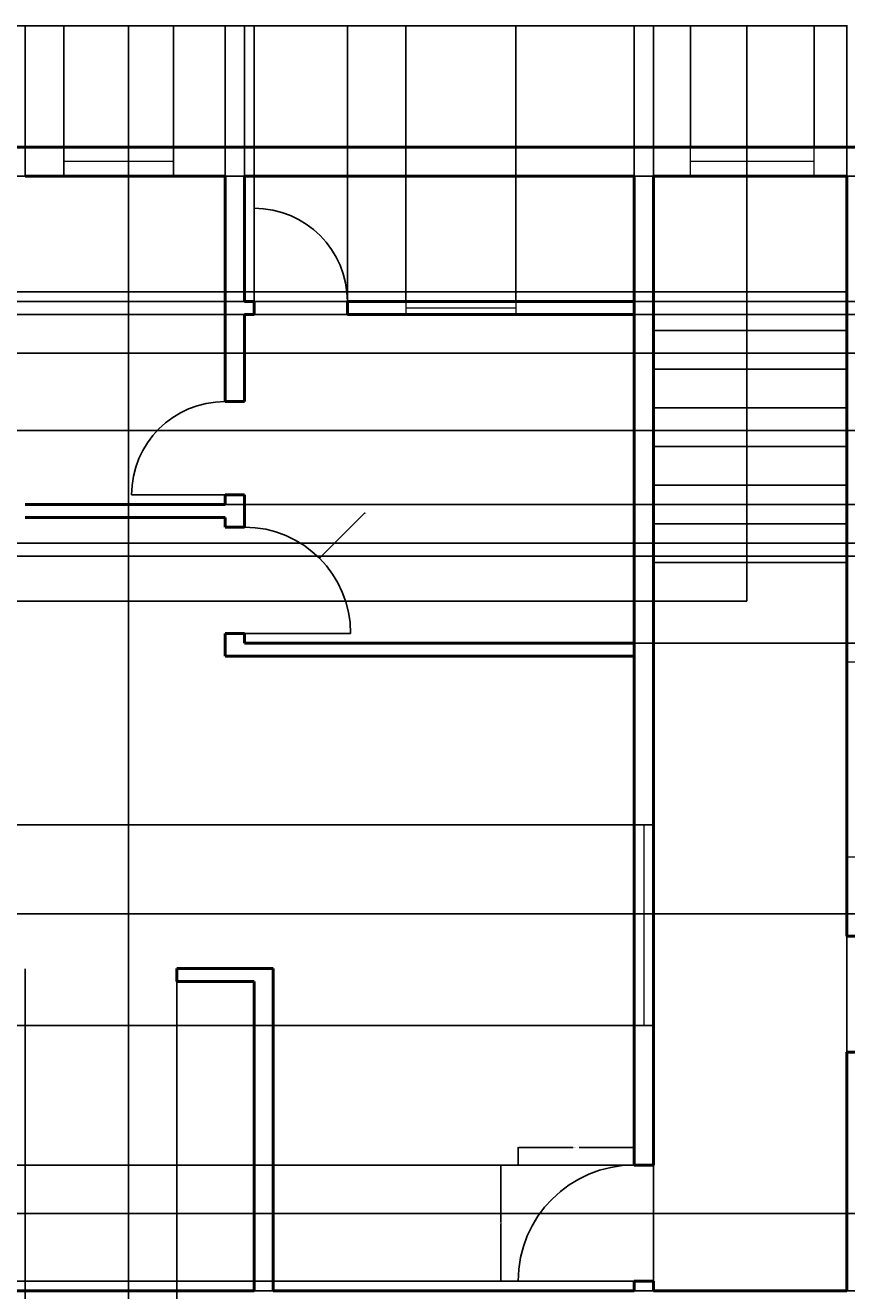
# Model space of a CAD drawing. Units: inches. Extents: x 2479 to 3284, y 2154 to 2936.
# Tile 4 of 8: x 2650 to 2905, y 2543 to 2936. Entities that reach past the tile are written whole.
import ezdxf

# ---------------------------------------------------------------- set-up
doc = ezdxf.new("R2010")
doc.units = ezdxf.units.IN
for name, color, linetype, lineweight in [('A-ANNO-DIMS', 2, 'Continuous', 18), ('A-DOOR', 3, 'Continuous', 25), ('A-FLOR-CASE', 8, 'Continuous', 18), ('A-FLOR-STRS', 2, 'Continuous', 25), ('A-GLAZ', 4, 'Continuous', 18), ('A-WALL', 7, 'Continuous', 50)]:
    doc.layers.add(name, color=color, linetype=linetype, lineweight=lineweight)
doc.styles.get("Standard").update_dxf_attribs({"font": 'arial.ttf'})
doc.dimstyles.get("Standard").update_dxf_attribs({"dimtxt": 0.18, "dimasz": 0.18, "dimexe": 0.18, "dimexo": 0.0625, "dimgap": 0.09, "dimtad": 0, "dimtih": 1, "dimtoh": 1, "dimdec": 4, "dimzin": 0, "dimdsep": 46, "dimtxsty": 'Standard', "dimcen": 0.09, "dimadec": 0, "dimazin": 0, "dimtfac": 1, "dimtdec": 4, "dimtofl": 0, "dimtmove": 0, "dimatfit": 3, "dimfxl": 1, "dimtolj": 1, "dimtzin": 0, "dimarcsym": 0})

# ---------------------------------------------------------------- blocks, each defined once
blk = doc.blocks.new('DOOR-SWING-29IN')
blk.add_line((29, 0), (0, 0))
blk.add_arc((29, 0), 29, 90, 180)
blk = doc.blocks.new('DOOR-SWING-36IN')
blk.add_line((36, 0), (0, 0))
blk.add_arc((36, 0), 36, 90, 180)
blk = doc.blocks.new('*D5')
at = {"layer": 'A-ANNO-DIMS', "color": 0, "lineweight": -2, "transparency": 16777216}
for p, q in [((2803.21, 2581.8), (2803.21, 2587.32)), ((2803.39, 2587.14), (2820.27, 2587.14)), ((2839.03, 2587.14), (2822.14, 2587.14)), ((2839.21, 2581.8), (2839.21, 2587.32))]:
    blk.add_line(p, q, dxfattribs=at)
at = {"layer": 'A-ANNO-DIMS', "color": 0, "transparency": 16777216}
for points in [[(2803.39, 2587.17), (2803.39, 2587.11), (2803.21, 2587.14)], [(2839.03, 2587.17), (2839.03, 2587.11), (2839.21, 2587.14)]]:
    blk.add_solid(points, dxfattribs=at)
at = {"layer": 'Defpoints', "color": 0, "transparency": 16777216}
for p in [(2839.21, 2587.14), (2803.21, 2581.74), (2839.21, 2581.74)]:
    blk.add_point(p, dxfattribs=at)
at = {"layer": 'A-ANNO-DIMS', "color": 0, "transparency": 16777216, "insert": (2821.21, 2587.14), "char_height": 0.18, "attachment_point": 5}
blk.add_mtext('\\A1;DOOR 36 TYP.', dxfattribs=at)
blk = doc.blocks.new('*D6')
at = {"layer": 'A-ANNO-DIMS', "color": 0, "lineweight": -2, "transparency": 16777216}
for p, q in [((2803.15, 2581.74), (2797.63, 2581.74)), ((2797.81, 2581.56), (2797.81, 2563.92)), ((2797.81, 2545.92), (2797.81, 2563.56)), ((2803.15, 2545.74), (2797.63, 2545.74))]:
    blk.add_line(p, q, dxfattribs=at)
at = {"layer": 'A-ANNO-DIMS', "color": 0, "transparency": 16777216}
for points in [[(2797.78, 2581.56), (2797.84, 2581.56), (2797.81, 2581.74)], [(2797.78, 2545.92), (2797.84, 2545.92), (2797.81, 2545.74)]]:
    blk.add_solid(points, dxfattribs=at)
at = {"layer": 'Defpoints', "color": 0, "transparency": 16777216}
for p in [(2797.81, 2581.74), (2803.21, 2581.74), (2803.21, 2545.74)]:
    blk.add_point(p, dxfattribs=at)
at = {"layer": 'A-ANNO-DIMS', "color": 0, "transparency": 16777216, "insert": (2797.81, 2563.74), "char_height": 0.18, "attachment_point": 5}
blk.add_mtext('\\A1;36 TYP.', dxfattribs=at)
blk = doc.blocks.new('*D9')
at = {"layer": 'A-ANNO-DIMS', "color": 0, "lineweight": -2, "transparency": 16777216}
for p, q in [((2517.21, 2897.8), (2517.21, 2935.52)), ((2517.39, 2935.34), (2710.92, 2935.34)), ((2905.03, 2935.34), (2711.5, 2935.34)), ((2905.21, 2888.8), (2905.21, 2935.52))]:
    blk.add_line(p, q, dxfattribs=at)
at = {"layer": 'A-ANNO-DIMS', "color": 0, "transparency": 16777216}
for points in [[(2517.39, 2935.37), (2517.39, 2935.31), (2517.21, 2935.34)], [(2905.03, 2935.37), (2905.03, 2935.31), (2905.21, 2935.34)]]:
    blk.add_solid(points, dxfattribs=at)
at = {"layer": 'Defpoints', "color": 0, "transparency": 16777216}
for p in [(2905.21, 2935.34), (2517.21, 2897.74), (2905.21, 2888.74)]:
    blk.add_point(p, dxfattribs=at)
at = {"layer": 'A-ANNO-DIMS', "color": 0, "transparency": 16777216, "insert": (2711.21, 2935.34), "char_height": 0.18, "attachment_point": 5}
blk.add_mtext('\\A1;388', dxfattribs=at)
blk = doc.blocks.new('*D11')
at = {"layer": 'A-ANNO-DIMS', "color": 0, "lineweight": -2, "transparency": 16777216}
for p, q in [((2845.21, 2542.8), (2845.21, 2935.52)), ((2845.39, 2935.34), (2874.99, 2935.34)), ((2905.03, 2935.34), (2875.43, 2935.34)), ((2905.21, 2542.8), (2905.21, 2935.52))]:
    blk.add_line(p, q, dxfattribs=at)
at = {"layer": 'A-ANNO-DIMS', "color": 0, "transparency": 16777216}
for points in [[(2845.39, 2935.37), (2845.39, 2935.31), (2845.21, 2935.34)], [(2905.03, 2935.37), (2905.03, 2935.31), (2905.21, 2935.34)]]:
    blk.add_solid(points, dxfattribs=at)
at = {"layer": 'Defpoints', "color": 0, "transparency": 16777216}
for p in [(2905.21, 2935.34), (2845.21, 2542.74), (2905.21, 2542.74)]:
    blk.add_point(p, dxfattribs=at)
at = {"layer": 'A-ANNO-DIMS', "color": 0, "transparency": 16777216, "insert": (2875.21, 2935.34), "char_height": 0.18, "attachment_point": 5}
blk.add_mtext('\\A1;60', dxfattribs=at)
blk = doc.blocks.new('*D27')
at = {"layer": 'A-ANNO-DIMS', "color": 0, "lineweight": -2, "transparency": 16777216}
for p, q in [((2845.15, 2545.74), (2479.43, 2545.74)), ((2479.61, 2545.56), (2479.61, 2536.92)), ((2479.61, 2527.92), (2479.61, 2536.56)), ((2845.15, 2527.74), (2479.43, 2527.74))]:
    blk.add_line(p, q, dxfattribs=at)
at = {"layer": 'A-ANNO-DIMS', "color": 0, "transparency": 16777216}
for points in [[(2479.58, 2545.56), (2479.64, 2545.56), (2479.61, 2545.74)], [(2479.58, 2527.92), (2479.64, 2527.92), (2479.61, 2527.74)]]:
    blk.add_solid(points, dxfattribs=at)
at = {"layer": 'Defpoints', "color": 0, "transparency": 16777216}
for p in [(2479.61, 2545.74), (2845.21, 2545.74), (2845.21, 2527.74)]:
    blk.add_point(p, dxfattribs=at)
at = {"layer": 'A-ANNO-DIMS', "color": 0, "transparency": 16777216, "insert": (2479.61, 2536.74), "char_height": 0.18, "attachment_point": 5}
blk.add_mtext('\\A1;18', dxfattribs=at)
blk = doc.blocks.new('*D28')
at = {"layer": 'A-ANNO-DIMS', "color": 0, "lineweight": -2, "transparency": 16777216}
for p, q in [((2845.15, 2625.04), (2479.43, 2625.04)), ((2479.61, 2624.86), (2479.61, 2603.57)), ((2479.61, 2581.92), (2479.61, 2603.21)), ((2845.15, 2581.74), (2479.43, 2581.74))]:
    blk.add_line(p, q, dxfattribs=at)
at = {"layer": 'A-ANNO-DIMS', "color": 0, "transparency": 16777216}
for points in [[(2479.58, 2624.86), (2479.64, 2624.86), (2479.61, 2625.04)], [(2479.58, 2581.92), (2479.64, 2581.92), (2479.61, 2581.74)]]:
    blk.add_solid(points, dxfattribs=at)
at = {"layer": 'Defpoints', "color": 0, "transparency": 16777216}
for p in [(2479.61, 2625.04), (2845.21, 2625.04), (2845.21, 2581.74)]:
    blk.add_point(p, dxfattribs=at)
at = {"layer": 'A-ANNO-DIMS', "color": 0, "transparency": 16777216, "insert": (2479.61, 2603.39), "char_height": 0.18, "attachment_point": 5}
blk.add_mtext('\\A1;43.3', dxfattribs=at)
blk = doc.blocks.new('*D29')
at = {"layer": 'A-ANNO-DIMS', "color": 0, "lineweight": -2, "transparency": 16777216}
for p, q in [((2845.15, 2687.36), (2479.43, 2687.36)), ((2479.61, 2687.18), (2479.61, 2656.38)), ((2479.61, 2625.22), (2479.61, 2656.01)), ((2845.15, 2625.04), (2479.43, 2625.04))]:
    blk.add_line(p, q, dxfattribs=at)
at = {"layer": 'A-ANNO-DIMS', "color": 0, "transparency": 16777216}
for points in [[(2479.58, 2687.18), (2479.64, 2687.18), (2479.61, 2687.36)], [(2479.58, 2625.22), (2479.64, 2625.22), (2479.61, 2625.04)]]:
    blk.add_solid(points, dxfattribs=at)
at = {"layer": 'Defpoints', "color": 0, "transparency": 16777216}
for p in [(2479.61, 2687.36), (2845.21, 2687.36), (2845.21, 2625.04)]:
    blk.add_point(p, dxfattribs=at)
at = {"layer": 'A-ANNO-DIMS', "color": 0, "transparency": 16777216, "insert": (2479.61, 2656.2), "char_height": 0.18, "attachment_point": 5}
blk.add_mtext('\\A1;62.32', dxfattribs=at)
blk = doc.blocks.new('*D30')
at = {"layer": 'A-ANNO-DIMS', "color": 0, "lineweight": -2, "transparency": 16777216}
for p, q in [((2845.15, 2852.74), (2479.43, 2852.74)), ((2479.61, 2852.56), (2479.61, 2804.92)), ((2479.61, 2756.92), (2479.61, 2804.56)), ((2845.15, 2756.74), (2479.43, 2756.74))]:
    blk.add_line(p, q, dxfattribs=at)
at = {"layer": 'A-ANNO-DIMS', "color": 0, "transparency": 16777216}
for points in [[(2479.58, 2852.56), (2479.64, 2852.56), (2479.61, 2852.74)], [(2479.58, 2756.92), (2479.64, 2756.92), (2479.61, 2756.74)]]:
    blk.add_solid(points, dxfattribs=at)
at = {"layer": 'Defpoints', "color": 0, "transparency": 16777216}
for p in [(2479.61, 2852.74), (2845.21, 2852.74), (2845.21, 2756.74)]:
    blk.add_point(p, dxfattribs=at)
at = {"layer": 'A-ANNO-DIMS', "color": 0, "transparency": 16777216, "insert": (2479.61, 2804.74), "char_height": 0.18, "attachment_point": 5}
blk.add_mtext('\\A1;96', dxfattribs=at)
blk = doc.blocks.new('*D31')
at = {"layer": 'A-ANNO-DIMS', "color": 0, "lineweight": -2, "transparency": 16777216}
for p, q in [((2845.15, 2888.74), (2479.43, 2888.74)), ((2479.61, 2888.56), (2479.61, 2870.92)), ((2479.61, 2852.92), (2479.61, 2870.56)), ((2845.15, 2852.74), (2479.43, 2852.74))]:
    blk.add_line(p, q, dxfattribs=at)
at = {"layer": 'A-ANNO-DIMS', "color": 0, "transparency": 16777216}
for points in [[(2479.58, 2888.56), (2479.64, 2888.56), (2479.61, 2888.74)], [(2479.58, 2852.92), (2479.64, 2852.92), (2479.61, 2852.74)]]:
    blk.add_solid(points, dxfattribs=at)
at = {"layer": 'Defpoints', "color": 0, "transparency": 16777216}
for p in [(2479.61, 2888.74), (2845.21, 2888.74), (2845.21, 2852.74)]:
    blk.add_point(p, dxfattribs=at)
at = {"layer": 'A-ANNO-DIMS', "color": 0, "transparency": 16777216, "insert": (2479.61, 2870.74), "char_height": 0.18, "attachment_point": 5}
blk.add_mtext('\\A1;36', dxfattribs=at)
blk = doc.blocks.new('*D33')
at = {"layer": 'A-ANNO-DIMS', "color": 0, "lineweight": -2, "transparency": 16777216}
for p, q in [((2845.21, 2756.8), (2845.21, 2935.52)), ((2845.39, 2935.34), (2859.49, 2935.34)), ((2874.03, 2935.34), (2859.93, 2935.34)), ((2874.21, 2756.8), (2874.21, 2935.52))]:
    blk.add_line(p, q, dxfattribs=at)
at = {"layer": 'A-ANNO-DIMS', "color": 0, "transparency": 16777216}
for points in [[(2845.39, 2935.37), (2845.39, 2935.31), (2845.21, 2935.34)], [(2874.03, 2935.37), (2874.03, 2935.31), (2874.21, 2935.34)]]:
    blk.add_solid(points, dxfattribs=at)
at = {"layer": 'Defpoints', "color": 0, "transparency": 16777216}
for p in [(2874.21, 2935.34), (2845.21, 2756.74), (2874.21, 2756.74)]:
    blk.add_point(p, dxfattribs=at)
at = {"layer": 'A-ANNO-DIMS', "color": 0, "transparency": 16777216, "insert": (2859.71, 2935.34), "char_height": 0.18, "attachment_point": 5}
blk.add_mtext('\\A1;29', dxfattribs=at)
blk = doc.blocks.new('*D34')
at = {"layer": 'A-ANNO-DIMS', "color": 0, "lineweight": -2, "transparency": 16777216}
for p, q in [((2856.82, 2897.74), (3283.99, 2897.74)), ((3283.81, 2897.56), (3283.81, 2893.42)), ((3283.81, 2888.92), (3283.81, 2893.06)), ((2856.82, 2888.74), (3283.99, 2888.74))]:
    blk.add_line(p, q, dxfattribs=at)
at = {"layer": 'A-ANNO-DIMS', "color": 0, "transparency": 16777216}
for points in [[(3283.78, 2897.56), (3283.84, 2897.56), (3283.81, 2897.74)], [(3283.78, 2888.92), (3283.84, 2888.92), (3283.81, 2888.74)]]:
    blk.add_solid(points, dxfattribs=at)
at = {"layer": 'Defpoints', "color": 0, "transparency": 16777216}
for p in [(2856.76, 2897.74), (3283.81, 2897.74), (2856.76, 2888.74)]:
    blk.add_point(p, dxfattribs=at)
at = {"layer": 'A-ANNO-DIMS', "color": 0, "transparency": 16777216, "insert": (3283.81, 2893.24), "char_height": 0.18, "attachment_point": 5}
blk.add_mtext('\\A1;9', dxfattribs=at)
blk = doc.blocks.new('*D35')
at = {"layer": 'A-ANNO-DIMS', "color": 0, "lineweight": -2, "transparency": 16777216}
for p, q in [((2845.21, 2888.8), (2845.21, 2935.52)), ((2845.39, 2935.34), (2850.53, 2935.34)), ((2856.58, 2935.34), (2851.44, 2935.34)), ((2856.76, 2897.8), (2856.76, 2935.52))]:
    blk.add_line(p, q, dxfattribs=at)
at = {"layer": 'A-ANNO-DIMS', "color": 0, "transparency": 16777216}
for points in [[(2845.39, 2935.37), (2845.39, 2935.31), (2845.21, 2935.34)], [(2856.58, 2935.37), (2856.58, 2935.31), (2856.76, 2935.34)]]:
    blk.add_solid(points, dxfattribs=at)
at = {"layer": 'Defpoints', "color": 0, "transparency": 16777216}
for p in [(2856.76, 2935.34), (2856.76, 2897.74), (2845.21, 2888.74)]:
    blk.add_point(p, dxfattribs=at)
at = {"layer": 'A-ANNO-DIMS', "color": 0, "transparency": 16777216, "insert": (2850.99, 2935.34), "char_height": 0.18, "attachment_point": 5}
blk.add_mtext('\\A1;11.553', dxfattribs=at)
blk = doc.blocks.new('*D36')
at = {"layer": 'A-ANNO-DIMS', "color": 0, "lineweight": -2, "transparency": 16777216}
for p, q in [((2856.76, 2897.8), (2856.76, 2935.52)), ((2856.94, 2935.34), (2875.55, 2935.34)), ((2894.95, 2935.34), (2876.34, 2935.34)), ((2895.13, 2897.8), (2895.13, 2935.52))]:
    blk.add_line(p, q, dxfattribs=at)
at = {"layer": 'A-ANNO-DIMS', "color": 0, "transparency": 16777216}
for points in [[(2856.94, 2935.37), (2856.94, 2935.31), (2856.76, 2935.34)], [(2894.95, 2935.37), (2894.95, 2935.31), (2895.13, 2935.34)]]:
    blk.add_solid(points, dxfattribs=at)
at = {"layer": 'Defpoints', "color": 0, "transparency": 16777216}
for p in [(2895.13, 2935.34), (2856.76, 2897.74), (2895.13, 2897.74)]:
    blk.add_point(p, dxfattribs=at)
at = {"layer": 'A-ANNO-DIMS', "color": 0, "transparency": 16777216, "insert": (2875.95, 2935.34), "char_height": 0.18, "attachment_point": 5}
blk.add_mtext('\\A1;38.37', dxfattribs=at)
blk = doc.blocks.new('*D40')
at = {"layer": 'A-ANNO-DIMS', "color": 0, "lineweight": -2, "transparency": 16777216}
for p, q in [((2646.21, 2888.8), (2646.21, 2935.52)), ((2646.39, 2935.34), (2648.06, 2935.34)), ((2650.03, 2935.34), (2648.36, 2935.34)), ((2650.21, 2888.8), (2650.21, 2935.52))]:
    blk.add_line(p, q, dxfattribs=at)
at = {"layer": 'A-ANNO-DIMS', "color": 0, "transparency": 16777216}
for points in [[(2646.39, 2935.37), (2646.39, 2935.31), (2646.21, 2935.34)], [(2650.03, 2935.37), (2650.03, 2935.31), (2650.21, 2935.34)]]:
    blk.add_solid(points, dxfattribs=at)
at = {"layer": 'Defpoints', "color": 0, "transparency": 16777216}
for p in [(2650.21, 2935.34), (2646.21, 2888.74), (2650.21, 2888.74)]:
    blk.add_point(p, dxfattribs=at)
at = {"layer": 'A-ANNO-DIMS', "color": 0, "transparency": 16777216, "insert": (2648.21, 2935.34), "char_height": 0.18, "attachment_point": 5}
blk.add_mtext('\\A1;4', dxfattribs=at)
blk = doc.blocks.new('*D41')
at = {"layer": 'A-ANNO-DIMS', "color": 0, "lineweight": -2, "transparency": 16777216}
for p, q in [((2650.21, 2888.8), (2650.21, 2935.52)), ((2650.39, 2935.34), (2655.74, 2935.34)), ((2661.99, 2935.34), (2656.64, 2935.34)), ((2662.17, 2888.8), (2662.17, 2935.52))]:
    blk.add_line(p, q, dxfattribs=at)
at = {"layer": 'A-ANNO-DIMS', "color": 0, "transparency": 16777216}
for points in [[(2650.39, 2935.37), (2650.39, 2935.31), (2650.21, 2935.34)], [(2661.99, 2935.37), (2661.99, 2935.31), (2662.17, 2935.34)]]:
    blk.add_solid(points, dxfattribs=at)
at = {"layer": 'Defpoints', "color": 0, "transparency": 16777216}
for p in [(2662.17, 2935.34), (2650.21, 2888.74), (2662.17, 2888.74)]:
    blk.add_point(p, dxfattribs=at)
at = {"layer": 'A-ANNO-DIMS', "color": 0, "transparency": 16777216, "insert": (2656.19, 2935.34), "char_height": 0.18, "attachment_point": 5}
blk.add_mtext('\\A1;11.962', dxfattribs=at)
blk = doc.blocks.new('*D42')
at = {"layer": 'A-ANNO-DIMS', "color": 0, "lineweight": -2, "transparency": 16777216}
for p, q in [((2662.17, 2888.8), (2662.17, 2935.52)), ((2662.35, 2935.34), (2678.74, 2935.34)), ((2696.05, 2935.34), (2679.67, 2935.34)), ((2696.23, 2888.8), (2696.23, 2935.52))]:
    blk.add_line(p, q, dxfattribs=at)
at = {"layer": 'A-ANNO-DIMS', "color": 0, "transparency": 16777216}
for points in [[(2662.35, 2935.37), (2662.35, 2935.31), (2662.17, 2935.34)], [(2696.05, 2935.37), (2696.05, 2935.31), (2696.23, 2935.34)]]:
    blk.add_solid(points, dxfattribs=at)
at = {"layer": 'Defpoints', "color": 0, "transparency": 16777216}
for p in [(2696.23, 2935.34), (2662.17, 2888.74), (2696.23, 2888.74)]:
    blk.add_point(p, dxfattribs=at)
at = {"layer": 'A-ANNO-DIMS', "color": 0, "transparency": 16777216, "insert": (2679.2, 2935.34), "char_height": 0.18, "attachment_point": 5}
blk.add_mtext('\\A1;34.064', dxfattribs=at)
blk = doc.blocks.new('*D43')
at = {"layer": 'A-ANNO-DIMS', "color": 0, "lineweight": -2, "transparency": 16777216}
for p, q in [((2696.23, 2888.8), (2696.23, 2935.52)), ((2696.41, 2935.34), (2703.77, 2935.34)), ((2712.03, 2935.34), (2704.68, 2935.34)), ((2712.21, 2888.8), (2712.21, 2935.52))]:
    blk.add_line(p, q, dxfattribs=at)
at = {"layer": 'A-ANNO-DIMS', "color": 0, "transparency": 16777216}
for points in [[(2696.41, 2935.37), (2696.41, 2935.31), (2696.23, 2935.34)], [(2712.03, 2935.37), (2712.03, 2935.31), (2712.21, 2935.34)]]:
    blk.add_solid(points, dxfattribs=at)
at = {"layer": 'Defpoints', "color": 0, "transparency": 16777216}
for p in [(2712.21, 2935.34), (2696.23, 2888.74), (2712.21, 2888.74)]:
    blk.add_point(p, dxfattribs=at)
at = {"layer": 'A-ANNO-DIMS', "color": 0, "transparency": 16777216, "insert": (2704.22, 2935.34), "char_height": 0.18, "attachment_point": 5}
blk.add_mtext('\\A1;15.975', dxfattribs=at)
blk = doc.blocks.new('*D44')
at = {"layer": 'A-ANNO-DIMS', "color": 0, "lineweight": -2, "transparency": 16777216}
for p, q in [((2718.21, 2849.8), (2718.21, 2935.52)), ((2718.39, 2935.34), (2719.56, 2935.34)), ((2721.03, 2935.34), (2719.86, 2935.34)), ((2721.21, 2849.8), (2721.21, 2935.52))]:
    blk.add_line(p, q, dxfattribs=at)
at = {"layer": 'A-ANNO-DIMS', "color": 0, "transparency": 16777216}
for points in [[(2718.39, 2935.37), (2718.39, 2935.31), (2718.21, 2935.34)], [(2721.03, 2935.37), (2721.03, 2935.31), (2721.21, 2935.34)]]:
    blk.add_solid(points, dxfattribs=at)
at = {"layer": 'Defpoints', "color": 0, "transparency": 16777216}
for p in [(2721.21, 2935.34), (2718.21, 2849.74), (2721.21, 2849.74)]:
    blk.add_point(p, dxfattribs=at)
at = {"layer": 'A-ANNO-DIMS', "color": 0, "transparency": 16777216, "insert": (2719.71, 2935.34), "char_height": 0.18, "attachment_point": 5}
blk.add_mtext('\\A1;3', dxfattribs=at)
blk = doc.blocks.new('*D45')
at = {"layer": 'A-ANNO-DIMS', "color": 0, "lineweight": -2, "transparency": 16777216}
for p, q in [((2750.21, 2849.8), (2750.21, 2935.52)), ((2750.39, 2935.34), (2758.89, 2935.34)), ((2768.17, 2935.34), (2759.66, 2935.34)), ((2768.35, 2849.8), (2768.35, 2935.52))]:
    blk.add_line(p, q, dxfattribs=at)
at = {"layer": 'A-ANNO-DIMS', "color": 0, "transparency": 16777216}
for points in [[(2750.39, 2935.37), (2750.39, 2935.31), (2750.21, 2935.34)], [(2768.17, 2935.37), (2768.17, 2935.31), (2768.35, 2935.34)]]:
    blk.add_solid(points, dxfattribs=at)
at = {"layer": 'Defpoints', "color": 0, "transparency": 16777216}
for p in [(2768.35, 2935.34), (2750.21, 2849.74), (2768.35, 2849.74)]:
    blk.add_point(p, dxfattribs=at)
at = {"layer": 'A-ANNO-DIMS', "color": 0, "transparency": 16777216, "insert": (2759.28, 2935.34), "char_height": 0.18, "attachment_point": 5}
blk.add_mtext('\\A1;18.14', dxfattribs=at)
blk = doc.blocks.new('*D46')
at = {"layer": 'A-ANNO-DIMS', "color": 0, "lineweight": -2, "transparency": 16777216}
for p, q in [((2768.35, 2849.8), (2768.35, 2935.52)), ((2768.53, 2935.34), (2784.95, 2935.34)), ((2802.3, 2935.34), (2785.88, 2935.34)), ((2802.48, 2849.8), (2802.48, 2935.52))]:
    blk.add_line(p, q, dxfattribs=at)
at = {"layer": 'A-ANNO-DIMS', "color": 0, "transparency": 16777216}
for points in [[(2768.53, 2935.37), (2768.53, 2935.31), (2768.35, 2935.34)], [(2802.3, 2935.37), (2802.3, 2935.31), (2802.48, 2935.34)]]:
    blk.add_solid(points, dxfattribs=at)
at = {"layer": 'Defpoints', "color": 0, "transparency": 16777216}
for p in [(2802.48, 2935.34), (2768.35, 2849.74), (2802.48, 2849.74)]:
    blk.add_point(p, dxfattribs=at)
at = {"layer": 'A-ANNO-DIMS', "color": 0, "transparency": 16777216, "insert": (2785.41, 2935.34), "char_height": 0.18, "attachment_point": 5}
blk.add_mtext('\\A1;34.126', dxfattribs=at)
blk = doc.blocks.new('*D47')
at = {"layer": 'A-ANNO-DIMS', "color": 0, "lineweight": -2, "transparency": 16777216}
for p, q in [((2802.48, 2849.8), (2802.48, 2935.52)), ((2802.66, 2935.34), (2820.45, 2935.34)), ((2839.03, 2935.34), (2821.24, 2935.34)), ((2839.21, 2849.8), (2839.21, 2935.52))]:
    blk.add_line(p, q, dxfattribs=at)
at = {"layer": 'A-ANNO-DIMS', "color": 0, "transparency": 16777216}
for points in [[(2802.66, 2935.37), (2802.66, 2935.31), (2802.48, 2935.34)], [(2839.03, 2935.37), (2839.03, 2935.31), (2839.21, 2935.34)]]:
    blk.add_solid(points, dxfattribs=at)
at = {"layer": 'Defpoints', "color": 0, "transparency": 16777216}
for p in [(2839.21, 2935.34), (2802.48, 2849.74), (2839.21, 2849.74)]:
    blk.add_point(p, dxfattribs=at)
at = {"layer": 'A-ANNO-DIMS', "color": 0, "transparency": 16777216, "insert": (2820.84, 2935.34), "char_height": 0.18, "attachment_point": 5}
blk.add_mtext('\\A1;36.73', dxfattribs=at)
blk = doc.blocks.new('*D58')
at = {"layer": 'A-ANNO-DIMS', "color": 0, "lineweight": -2, "transparency": 16777216}
for p, q in [((2718.27, 2888.74), (3283.99, 2888.74)), ((3283.81, 2888.56), (3283.81, 2869.42)), ((3283.81, 2849.92), (3283.81, 2869.06)), ((2718.27, 2849.74), (3283.99, 2849.74))]:
    blk.add_line(p, q, dxfattribs=at)
at = {"layer": 'A-ANNO-DIMS', "color": 0, "transparency": 16777216}
for points in [[(3283.78, 2888.56), (3283.84, 2888.56), (3283.81, 2888.74)], [(3283.78, 2849.92), (3283.84, 2849.92), (3283.81, 2849.74)]]:
    blk.add_solid(points, dxfattribs=at)
at = {"layer": 'Defpoints', "color": 0, "transparency": 16777216}
for p in [(2718.21, 2888.74), (3283.81, 2888.74), (2718.21, 2849.74)]:
    blk.add_point(p, dxfattribs=at)
at = {"layer": 'A-ANNO-DIMS', "color": 0, "transparency": 16777216, "insert": (3283.81, 2869.24), "char_height": 0.18, "attachment_point": 5}
blk.add_mtext('\\A1;39', dxfattribs=at)
blk = doc.blocks.new('*D59')
at = {"layer": 'A-ANNO-DIMS', "color": 0, "lineweight": -2, "transparency": 16777216}
for p, q in [((2839.27, 2845.74), (3283.99, 2845.74)), ((3283.81, 2845.56), (3283.81, 2816.42)), ((3283.81, 2786.92), (3283.81, 2816.06)), ((2712.27, 2786.74), (3283.99, 2786.74))]:
    blk.add_line(p, q, dxfattribs=at)
at = {"layer": 'A-ANNO-DIMS', "color": 0, "transparency": 16777216}
for points in [[(3283.78, 2845.56), (3283.84, 2845.56), (3283.81, 2845.74)], [(3283.78, 2786.92), (3283.84, 2786.92), (3283.81, 2786.74)]]:
    blk.add_solid(points, dxfattribs=at)
at = {"layer": 'Defpoints', "color": 0, "transparency": 16777216}
for p in [(2839.21, 2845.74), (3283.81, 2845.74), (2712.21, 2786.74)]:
    blk.add_point(p, dxfattribs=at)
at = {"layer": 'A-ANNO-DIMS', "color": 0, "transparency": 16777216, "insert": (3283.81, 2816.24), "char_height": 0.18, "attachment_point": 5}
blk.add_mtext('\\A1;59', dxfattribs=at)
blk = doc.blocks.new('*D60')
at = {"layer": 'A-ANNO-DIMS', "color": 0, "lineweight": -2, "transparency": 16777216}
for p, q in [((2712.27, 2786.74), (3283.99, 2786.74)), ((3283.81, 2786.56), (3283.81, 2765.42)), ((3283.81, 2743.92), (3283.81, 2765.06)), ((2839.27, 2743.74), (3283.99, 2743.74))]:
    blk.add_line(p, q, dxfattribs=at)
at = {"layer": 'A-ANNO-DIMS', "color": 0, "transparency": 16777216}
for points in [[(3283.78, 2786.56), (3283.84, 2786.56), (3283.81, 2786.74)], [(3283.78, 2743.92), (3283.84, 2743.92), (3283.81, 2743.74)]]:
    blk.add_solid(points, dxfattribs=at)
at = {"layer": 'Defpoints', "color": 0, "transparency": 16777216}
for p in [(2712.21, 2786.74), (3283.81, 2786.74), (2839.21, 2743.74)]:
    blk.add_point(p, dxfattribs=at)
at = {"layer": 'A-ANNO-DIMS', "color": 0, "transparency": 16777216, "insert": (3283.81, 2765.24), "char_height": 0.18, "attachment_point": 5}
blk.add_mtext('\\A1;43', dxfattribs=at)
blk = doc.blocks.new('*D61')
at = {"layer": 'A-ANNO-DIMS', "color": 0, "lineweight": -2, "transparency": 16777216}
for p, q in [((2595.27, 2566.74), (3283.99, 2566.74)), ((3283.81, 2566.56), (3283.81, 2554.92)), ((3283.81, 2542.92), (3283.81, 2554.56)), ((2595.27, 2542.74), (3283.99, 2542.74))]:
    blk.add_line(p, q, dxfattribs=at)
at = {"layer": 'A-ANNO-DIMS', "color": 0, "transparency": 16777216}
for points in [[(3283.78, 2566.56), (3283.84, 2566.56), (3283.81, 2566.74)], [(3283.78, 2542.92), (3283.84, 2542.92), (3283.81, 2542.74)]]:
    blk.add_solid(points, dxfattribs=at)
at = {"layer": 'Defpoints', "color": 0, "transparency": 16777216}
for p in [(2595.21, 2566.74), (3283.81, 2566.74), (2595.21, 2542.74)]:
    blk.add_point(p, dxfattribs=at)
at = {"layer": 'A-ANNO-DIMS', "color": 0, "transparency": 16777216, "insert": (3283.81, 2554.74), "char_height": 0.18, "attachment_point": 5}
blk.add_mtext('\\A1;24', dxfattribs=at)
blk = doc.blocks.new('*D63')
at = {"layer": 'A-ANNO-DIMS', "color": 0, "lineweight": -2, "transparency": 16777216}
for p, q in [((2650.21, 2642.68), (2650.21, 2153.96)), ((2697.21, 2642.68), (2697.21, 2153.96)), ((2650.39, 2154.14), (2673.49, 2154.14)), ((2697.03, 2154.14), (2673.93, 2154.14))]:
    blk.add_line(p, q, dxfattribs=at)
at = {"layer": 'A-ANNO-DIMS', "color": 0, "transparency": 16777216}
for points in [[(2650.39, 2154.17), (2650.39, 2154.11), (2650.21, 2154.14)], [(2697.03, 2154.17), (2697.03, 2154.11), (2697.21, 2154.14)]]:
    blk.add_solid(points, dxfattribs=at)
at = {"layer": 'Defpoints', "color": 0, "transparency": 16777216}
for p in [(2650.21, 2642.74), (2697.21, 2642.74), (2697.21, 2154.14)]:
    blk.add_point(p, dxfattribs=at)
at = {"layer": 'A-ANNO-DIMS', "color": 0, "transparency": 16777216, "insert": (2673.71, 2154.14), "char_height": 0.18, "attachment_point": 5}
blk.add_mtext('\\A1;47', dxfattribs=at)
blk = doc.blocks.new('*D84')
at = {"layer": 'A-ANNO-DIMS', "color": 0, "lineweight": -2, "transparency": 16777216}
for p, q in [((3032.15, 2888.74), (2479.43, 2888.74)), ((2479.61, 2888.56), (2479.61, 2869.42)), ((2479.61, 2849.92), (2479.61, 2869.06)), ((3032.15, 2849.74), (2479.43, 2849.74))]:
    blk.add_line(p, q, dxfattribs=at)
at = {"layer": 'A-ANNO-DIMS', "color": 0, "transparency": 16777216}
for points in [[(2479.58, 2888.56), (2479.64, 2888.56), (2479.61, 2888.74)], [(2479.58, 2849.92), (2479.64, 2849.92), (2479.61, 2849.74)]]:
    blk.add_solid(points, dxfattribs=at)
at = {"layer": 'Defpoints', "color": 0, "transparency": 16777216}
for p in [(2479.61, 2888.74), (3032.21, 2888.74), (3032.21, 2849.74)]:
    blk.add_point(p, dxfattribs=at)
at = {"layer": 'A-ANNO-DIMS', "color": 0, "transparency": 16777216, "insert": (2479.61, 2869.24), "char_height": 0.18, "attachment_point": 5}
blk.add_mtext('\\A1;39', dxfattribs=at)
blk = doc.blocks.new('*D85')
at = {"layer": 'A-ANNO-DIMS', "color": 0, "lineweight": -2, "transparency": 16777216}
for p, q in [((2911.15, 2845.74), (2479.43, 2845.74)), ((2479.61, 2845.56), (2479.61, 2810.42)), ((2479.61, 2774.92), (2479.61, 2810.06)), ((3041.15, 2774.74), (2479.43, 2774.74))]:
    blk.add_line(p, q, dxfattribs=at)
at = {"layer": 'A-ANNO-DIMS', "color": 0, "transparency": 16777216}
for points in [[(2479.58, 2845.56), (2479.64, 2845.56), (2479.61, 2845.74)], [(2479.58, 2774.92), (2479.64, 2774.92), (2479.61, 2774.74)]]:
    blk.add_solid(points, dxfattribs=at)
at = {"layer": 'Defpoints', "color": 0, "transparency": 16777216}
for p in [(2479.61, 2845.74), (2911.21, 2845.74), (3041.21, 2774.74)]:
    blk.add_point(p, dxfattribs=at)
at = {"layer": 'A-ANNO-DIMS', "color": 0, "transparency": 16777216, "insert": (2479.61, 2810.24), "char_height": 0.18, "attachment_point": 5}
blk.add_mtext('\\A1;71', dxfattribs=at)
blk = doc.blocks.new('*D86')
at = {"layer": 'A-ANNO-DIMS', "color": 0, "lineweight": -2, "transparency": 16777216}
for p, q in [((3041.15, 2770.74), (2479.43, 2770.74)), ((2479.61, 2770.56), (2479.61, 2715.42)), ((2479.61, 2659.92), (2479.61, 2715.06)), ((2911.15, 2659.74), (2479.43, 2659.74))]:
    blk.add_line(p, q, dxfattribs=at)
at = {"layer": 'A-ANNO-DIMS', "color": 0, "transparency": 16777216}
for points in [[(2479.58, 2770.56), (2479.64, 2770.56), (2479.61, 2770.74)], [(2479.58, 2659.92), (2479.64, 2659.92), (2479.61, 2659.74)]]:
    blk.add_solid(points, dxfattribs=at)
at = {"layer": 'Defpoints', "color": 0, "transparency": 16777216}
for p in [(2479.61, 2770.74), (3041.21, 2770.74), (2911.21, 2659.74)]:
    blk.add_point(p, dxfattribs=at)
at = {"layer": 'A-ANNO-DIMS', "color": 0, "transparency": 16777216, "insert": (2479.61, 2715.24), "char_height": 0.18, "attachment_point": 5}
blk.add_mtext('\\A1;111', dxfattribs=at)
blk = doc.blocks.new('*D89')
at = {"layer": 'A-ANNO-DIMS', "color": 0, "lineweight": -2, "transparency": 16777216}
for p, q in [((3139.15, 2833.74), (2479.43, 2833.74)), ((2479.61, 2833.56), (2479.61, 2821.92)), ((2479.61, 2809.92), (2479.61, 2821.56)), ((3213.15, 2809.74), (2479.43, 2809.74))]:
    blk.add_line(p, q, dxfattribs=at)
at = {"layer": 'A-ANNO-DIMS', "color": 0, "transparency": 16777216}
for points in [[(2479.58, 2833.56), (2479.64, 2833.56), (2479.61, 2833.74)], [(2479.58, 2809.92), (2479.64, 2809.92), (2479.61, 2809.74)]]:
    blk.add_solid(points, dxfattribs=at)
at = {"layer": 'Defpoints', "color": 0, "transparency": 16777216}
for p in [(2479.61, 2833.74), (3139.21, 2833.74), (3213.21, 2809.74)]:
    blk.add_point(p, dxfattribs=at)
at = {"layer": 'A-ANNO-DIMS', "color": 0, "transparency": 16777216, "insert": (2479.61, 2821.74), "char_height": 0.18, "attachment_point": 5}
blk.add_mtext('\\A1;24', dxfattribs=at)
blk = doc.blocks.new('*D110')
at = {"layer": 'A-ANNO-DIMS', "color": 0, "lineweight": -2, "transparency": 16777216}
for p, q in [((2643.21, 2407.8), (2643.21, 2935.52)), ((2643.39, 2935.34), (2662.49, 2935.34)), ((2682.03, 2935.34), (2662.93, 2935.34)), ((2682.21, 2407.8), (2682.21, 2935.52))]:
    blk.add_line(p, q, dxfattribs=at)
at = {"layer": 'A-ANNO-DIMS', "color": 0, "transparency": 16777216}
for points in [[(2643.39, 2935.37), (2643.39, 2935.31), (2643.21, 2935.34)], [(2682.03, 2935.37), (2682.03, 2935.31), (2682.21, 2935.34)]]:
    blk.add_solid(points, dxfattribs=at)
at = {"layer": 'Defpoints', "color": 0, "transparency": 16777216}
for p in [(2682.21, 2935.34), (2643.21, 2407.74), (2682.21, 2407.74)]:
    blk.add_point(p, dxfattribs=at)
at = {"layer": 'A-ANNO-DIMS', "color": 0, "transparency": 16777216, "insert": (2662.71, 2935.34), "char_height": 0.18, "attachment_point": 5}
blk.add_mtext('\\A1;39', dxfattribs=at)
blk = doc.blocks.new('*D136')
at = {"layer": 'A-ANNO-DIMS', "color": 0, "lineweight": -2, "transparency": 16777216}
for p, q in [((2755.54, 2784.08), (2741.67, 2770.2)), ((2755.72, 2784.08), (2755.54, 2784.08)), ((2718.12, 2746.74), (2718.3, 2746.74)), ((2718.21, 2746.65), (2718.21, 2746.83))]:
    blk.add_line(p, q, dxfattribs=at)
at = {"layer": 'A-ANNO-DIMS', "color": 0, "transparency": 16777216}
blk.add_solid([(2741.65, 2770.22), (2741.69, 2770.18), (2741.54, 2770.07)], dxfattribs=at)
at = {"layer": 'Defpoints', "color": 0, "transparency": 16777216}
for p in [(2741.54, 2770.07), (2718.21, 2746.74)]:
    blk.add_point(p, dxfattribs=at)
at = {"layer": 'A-ANNO-DIMS', "color": 0, "transparency": 16777216, "insert": (2756.03, 2784.08), "char_height": 0.18, "attachment_point": 5}
blk.add_mtext('\\A1;R33', dxfattribs=at)

msp = doc.modelspace()

# ---------------------------------------------------------------- linework, layer by layer
at = {"layer": 'A-DOOR'}
msp.add_line((2718.2088, 2746.7397), (2751.2088, 2746.7397), dxfattribs=at)
msp.add_arc((2718.2088, 2746.7397), 33, 0, 90, dxfattribs=at)
at = {"layer": 'A-FLOR-CASE'}
for p, q in [((2697.2088, 2638.7397), (2697.2088, 2566.7397)), ((2697.2088, 2566.7397), (2595.2088, 2566.7397))]:
    msp.add_line(p, q, dxfattribs=at)
at = {"layer": 'A-FLOR-STRS'}
for p, q in [((2905.2088, 2852.7397), (2845.2088, 2852.7397)), ((2874.2088, 2852.7397), (2874.2088, 2756.7397)), ((2905.2088, 2840.7397), (2845.2088, 2840.7397)), ((2905.2088, 2828.7397), (2845.2088, 2828.7397)), ((2905.2088, 2816.7397), (2845.2088, 2816.7397)), ((2905.2088, 2804.7397), (2845.2088, 2804.7397)), ((2905.2088, 2792.7397), (2845.2088, 2792.7397)), ((2905.2088, 2780.7397), (2845.2088, 2780.7397)), ((2905.2088, 2768.7397), (2845.2088, 2768.7397)), ((2874.2088, 2756.7397), (2845.2088, 2756.7397))]:
    msp.add_line(p, q, dxfattribs=at)
at = {"layer": 'A-GLAZ'}
for p, q in [((2662.1708, 2888.7397), (2662.1708, 2897.7397)), ((2696.2343, 2888.7397), (2696.2343, 2897.7397)), ((2856.7618, 2888.7397), (2856.7618, 2897.7397)), ((2895.1321, 2888.7397), (2895.1321, 2897.7397)), ((2696.2343, 2893.2397), (2662.1708, 2893.2397)), ((2895.1321, 2893.2397), (2856.7618, 2893.2397)), ((2768.3501, 2849.7397), (2768.3501, 2845.7397)), ((2802.4758, 2847.7397), (2768.3501, 2847.7397)), ((2802.4758, 2849.7397), (2802.4758, 2845.7397)), ((2911.2088, 2737.8354), (2905.2088, 2737.8354)), ((2845.2088, 2687.3564), (2839.2088, 2687.3564)), ((2842.2088, 2687.3564), (2842.2088, 2625.0365)), ((2911.2088, 2677.3151), (2905.2088, 2677.3151)), ((2845.2088, 2625.0365), (2839.2088, 2625.0365))]:
    msp.add_line(p, q, dxfattribs=at)
at = {"layer": 'A-WALL'}
for p, q in [((3246.2088, 2897.7397), (2517.2088, 2897.7397)), ((2712.2088, 2888.7397), (2650.2088, 2888.7397)), ((2712.2088, 2888.7397), (2712.2088, 2818.7397)), ((2718.2088, 2888.7397), (2718.2088, 2849.7397)), ((2839.2088, 2888.7397), (2718.2088, 2888.7397)), ((2839.2088, 2888.7397), (2839.2088, 2581.7397)), ((2845.2088, 2888.7397), (2845.2088, 2581.7397)), ((2905.2088, 2888.7397), (2845.2088, 2888.7397)), ((2905.2088, 2888.7397), (2905.2088, 2652.7397)), ((2721.2088, 2849.7397), (2718.2088, 2849.7397)), ((2721.2088, 2849.7397), (2721.2088, 2845.7397)), ((2839.2088, 2849.7397), (2750.2088, 2849.7397)), ((2750.2088, 2849.7397), (2750.2088, 2845.7397)), ((2721.2088, 2845.7397), (2718.2088, 2845.7397)), ((2718.2088, 2845.7397), (2718.2088, 2818.7397)), ((2839.2088, 2845.7397), (2750.2088, 2845.7397)), ((2712.2088, 2818.7397), (2718.2088, 2818.7397)), ((2712.2088, 2789.7397), (2718.2088, 2789.7397)), ((2712.2088, 2789.7397), (2712.2088, 2786.7397)), ((2718.2088, 2789.7397), (2718.2088, 2779.7397)), ((2712.2088, 2786.7397), (2650.2088, 2786.7397)), ((2712.2088, 2782.7397), (2650.2088, 2782.7397)), ((2712.2088, 2782.7397), (2712.2088, 2779.7397)), ((2718.2088, 2779.7397), (2712.2088, 2779.7397)), ((2718.2088, 2746.7397), (2712.2088, 2746.7397)), ((2712.2088, 2746.7397), (2712.2088, 2739.7397)), ((2718.2088, 2746.7397), (2718.2088, 2743.7397)), ((2839.2088, 2743.7397), (2718.2088, 2743.7397)), ((2839.2088, 2739.7397), (2712.2088, 2739.7397)), ((2911.2088, 2652.7397), (2905.2088, 2652.7397)), ((2712.2088, 2642.7397), (2697.2088, 2642.7397)), ((2697.2088, 2642.7397), (2697.2088, 2638.7397)), ((2718.2088, 2642.7397), (2712.2088, 2642.7397)), ((2727.2088, 2642.7397), (2718.2088, 2642.7397)), ((2727.2088, 2638.7397), (2727.2088, 2642.7397)), ((2721.2088, 2638.7397), (2697.2088, 2638.7397)), ((2721.2088, 2638.7397), (2721.2088, 2542.7397)), ((2727.2088, 2638.7397), (2727.2088, 2542.7397)), ((2911.2088, 2616.7397), (2905.2088, 2616.7397)), ((2905.2088, 2616.7397), (2905.2088, 2542.7397)), ((2845.2088, 2581.7397), (2839.2088, 2581.7397)), ((2845.2088, 2545.7397), (2839.2088, 2545.7397)), ((2839.2088, 2545.7397), (2839.2088, 2542.7397)), ((2845.2088, 2545.7397), (2845.2088, 2542.7397)), ((2721.2088, 2542.7397), (2595.2088, 2542.7397)), ((2839.2088, 2542.7397), (2727.2088, 2542.7397)), ((2905.2088, 2542.7397), (2845.2088, 2542.7397))]:
    msp.add_line(p, q, dxfattribs=at)

# ---------------------------------------------------------------- block references
at = {"layer": 'A-DOOR', "rotation": 270}
msp.add_blockref('DOOR-SWING-29IN', (2721.2088, 2878.7397), dxfattribs=at)
at = {"layer": 'A-DOOR'}
for name, p in [('DOOR-SWING-29IN', (2683.2088, 2789.7397)), ('DOOR-SWING-36IN', (2803.2088, 2545.7397))]:
    msp.add_blockref(name, p, dxfattribs=at)

# ---------------------------------------------------------------- dimensions: what is measured, and where the dimension line sits
at = {"layer": 'A-ANNO-DIMS'}
for base, p1, p2, override, picture, middle in [((2905.2088, 2935.3397), (2517.2088, 2897.7397), (2905.2088, 2888.7397), {"dimdec": 0, "dimlfac": 1, "dimrnd": 0, "dimzin": 0, "dimdsep": 46, "dimlunit": 2}, '*D9', (2711.2088, 2935.3397)), ((2682.2088, 2935.3397), (2643.2088, 2407.7397), (2682.2088, 2407.7397), {"dimdec": 0, "dimlfac": 1, "dimrnd": 0, "dimzin": 0, "dimdsep": 46, "dimlunit": 2}, '*D110', (2662.7088, 2935.3397)), ((2650.2088, 2935.3397), (2646.2088, 2888.7397), (2650.2088, 2888.7397), {"dimdec": 0, "dimlfac": 1, "dimrnd": 0, "dimzin": 0, "dimdsep": 46, "dimlunit": 2}, '*D40', (2648.2088, 2935.3397)), ((2662.1708, 2935.3397), (2650.2088, 2888.7397), (2662.1708, 2888.7397), {"dimdec": 3, "dimlfac": 1, "dimrnd": 0, "dimzin": 0, "dimdsep": 46, "dimlunit": 2}, '*D41', (2656.1898, 2935.3397)), ((2696.2343, 2935.33975), (2662.17077, 2888.73975), (2696.2343, 2888.73975), {"dimdec": 3, "dimlfac": 1, "dimrnd": 0, "dimzin": 0, "dimdsep": 46, "dimlunit": 2}, '*D42', (2679.20253, 2935.33975)), ((2712.20882, 2935.33975), (2696.2343, 2888.73975), (2712.20882, 2888.73975), {"dimdec": 3, "dimlfac": 1, "dimrnd": 0, "dimzin": 0, "dimdsep": 46, "dimlunit": 2}, '*D43', (2704.22156, 2935.33975)), ((2721.2088, 2935.3397), (2718.2088, 2849.7397), (2721.2088, 2849.7397), {"dimdec": 0, "dimlfac": 1, "dimrnd": 0, "dimzin": 0, "dimdsep": 46, "dimlunit": 2}, '*D44', (2719.7088, 2935.3397)), ((2768.3501, 2935.3397), (2750.2088, 2849.7397), (2768.3501, 2849.7397), {"dimdec": 2, "dimlfac": 1, "dimrnd": 0, "dimzin": 0, "dimdsep": 46, "dimlunit": 2}, '*D45', (2759.2795, 2935.3397)), ((2802.4758, 2935.3397), (2768.3501, 2849.7397), (2802.4758, 2849.7397), {"dimdec": 3, "dimlfac": 1, "dimrnd": 0, "dimzin": 0, "dimdsep": 46, "dimlunit": 2}, '*D46', (2785.413, 2935.3397)), ((2839.2088, 2935.3397), (2802.4758, 2849.7397), (2839.2088, 2849.7397), {"dimdec": 2, "dimlfac": 1, "dimrnd": 0, "dimzin": 0, "dimdsep": 46, "dimlunit": 2}, '*D47', (2820.8423, 2935.3397)), ((2905.2088, 2935.3397), (2845.2088, 2542.7397), (2905.2088, 2542.7397), {"dimdec": 0, "dimlfac": 1, "dimrnd": 0, "dimzin": 0, "dimdsep": 46, "dimlunit": 2}, '*D11', (2875.2088, 2935.3397)), ((2874.2088, 2935.3397), (2845.2088, 2756.7397), (2874.2088, 2756.7397), {"dimdec": 0, "dimlfac": 1, "dimrnd": 0, "dimzin": 0, "dimdsep": 46, "dimlunit": 2}, '*D33', (2859.7088, 2935.3397)), ((2856.7618, 2935.3397), (2845.2088, 2888.7397), (2856.7618, 2897.7397), {"dimdec": 3, "dimlfac": 1, "dimrnd": 0, "dimzin": 0, "dimdsep": 46, "dimlunit": 2}, '*D35', (2850.9853, 2935.3397)), ((2895.1321, 2935.3397), (2856.7618, 2897.7397), (2895.1321, 2897.7397), {"dimdec": 2, "dimlfac": 1, "dimrnd": 0, "dimzin": 0, "dimdsep": 46, "dimlunit": 2}, '*D36', (2875.9469, 2935.3397)), ((2697.2088, 2154.1397), (2650.2088, 2642.7397), (2697.2088, 2642.7397), {"dimdec": 0, "dimlfac": 1, "dimrnd": 0, "dimzin": 0, "dimdsep": 46, "dimlunit": 2}, '*D63', (2673.7088, 2154.1397))]:
    dim = msp.add_linear_dim(base=base, p1=p1, p2=p2, dimstyle='Standard', override=override, dxfattribs=at)
    dim.commit()
    dim.dimension.update_dxf_attribs({"geometry": picture, "text_midpoint": middle})
for base, p1, p2, override, picture, middle in [((3283.8088, 2897.7397), (2856.7618, 2888.7397), (2856.7618, 2897.7397), {"dimdec": 0, "dimlfac": 1, "dimrnd": 0, "dimzin": 0, "dimdsep": 46, "dimlunit": 2}, '*D34', (3283.8088, 2893.2397)), ((2479.6088, 2888.7397), (2845.2088, 2852.7397), (2845.2088, 2888.7397), {"dimdec": 0, "dimlfac": 1, "dimrnd": 0, "dimzin": 0, "dimdsep": 46, "dimlunit": 2}, '*D31', (2479.6088, 2870.7397)), ((2479.6088, 2888.7397), (3032.2088, 2849.7397), (3032.2088, 2888.7397), {"dimdec": 0, "dimlfac": 1, "dimrnd": 0, "dimzin": 0, "dimdsep": 46, "dimlunit": 2}, '*D84', (2479.6088, 2869.2397)), ((3283.8088, 2888.7397), (2718.2088, 2849.7397), (2718.2088, 2888.7397), {"dimdec": 0, "dimlfac": 1, "dimrnd": 0, "dimzin": 0, "dimdsep": 46, "dimlunit": 2}, '*D58', (3283.8088, 2869.2397)), ((2479.6088, 2852.7397), (2845.2088, 2756.7397), (2845.2088, 2852.7397), {"dimdec": 0, "dimlfac": 1, "dimrnd": 0, "dimzin": 0, "dimdsep": 46, "dimlunit": 2}, '*D30', (2479.6088, 2804.7397)), ((2479.6088, 2845.7397), (3041.2088, 2774.7397), (2911.2088, 2845.7397), {"dimdec": 0, "dimlfac": 1, "dimrnd": 0, "dimzin": 0, "dimdsep": 46, "dimlunit": 2}, '*D85', (2479.6088, 2810.2397)), ((3283.8088, 2845.7397), (2712.2088, 2786.7397), (2839.2088, 2845.7397), {"dimdec": 0, "dimlfac": 1, "dimrnd": 0, "dimzin": 0, "dimdsep": 46, "dimlunit": 2}, '*D59', (3283.8088, 2816.2397)), ((2479.6088, 2833.7397), (3213.2088, 2809.7397), (3139.2088, 2833.7397), {"dimdec": 0, "dimlfac": 1, "dimrnd": 0, "dimzin": 0, "dimdsep": 46, "dimlunit": 2}, '*D89', (2479.6088, 2821.7397)), ((3283.8088, 2786.7397), (2839.2088, 2743.7397), (2712.2088, 2786.7397), {"dimdec": 0, "dimlfac": 1, "dimrnd": 0, "dimzin": 0, "dimdsep": 46, "dimlunit": 2}, '*D60', (3283.8088, 2765.2397)), ((2479.6088, 2770.7397), (2911.2088, 2659.7397), (3041.2088, 2770.7397), {"dimdec": 0, "dimlfac": 1, "dimrnd": 0, "dimzin": 0, "dimdsep": 46, "dimlunit": 2}, '*D86', (2479.6088, 2715.2397)), ((2479.6088, 2687.3564), (2845.2088, 2625.0365), (2845.2088, 2687.3564), {"dimdec": 2, "dimlfac": 1, "dimrnd": 0, "dimzin": 0, "dimdsep": 46, "dimlunit": 2}, '*D29', (2479.6088, 2656.1965)), ((2479.6088, 2625.0365), (2845.2088, 2581.7397), (2845.2088, 2625.0365), {"dimdec": 1, "dimlfac": 1, "dimrnd": 0, "dimzin": 0, "dimdsep": 46, "dimlunit": 2}, '*D28', (2479.6088, 2603.3881)), ((3283.8088, 2566.7397), (2595.2088, 2542.7397), (2595.2088, 2566.7397), {"dimdec": 0, "dimlfac": 1, "dimrnd": 0, "dimzin": 0, "dimdsep": 46, "dimlunit": 2}, '*D61', (3283.8088, 2554.7397)), ((2479.6088, 2545.7397), (2845.2088, 2527.7397), (2845.2088, 2545.7397), {"dimdec": 0, "dimlfac": 1, "dimrnd": 0, "dimzin": 0, "dimdsep": 46, "dimlunit": 2}, '*D27', (2479.6088, 2536.7397))]:
    dim = msp.add_linear_dim(base=base, p1=p1, p2=p2, angle=90, dimstyle='Standard', override=override, dxfattribs=at)
    dim.commit()
    dim.dimension.update_dxf_attribs({"geometry": picture, "text_midpoint": middle})
dim = msp.add_radius_dim(center=(2718.2088, 2746.7397), mpoint=(2741.5433, 2770.0743), dimstyle='Standard', override={"dimdec": 0, "dimlfac": 1, "dimrnd": 0, "dimzin": 0, "dimdsep": 46, "dimlunit": 2}, dxfattribs=at)
dim.commit()
dim.dimension.update_dxf_attribs({"geometry": '*D136', "text_midpoint": (2756.0291, 2784.075), "dimtype": 164})
dim = msp.add_linear_dim(base=(2839.2088, 2587.1397), p1=(2803.2088, 2581.7397), p2=(2839.2088, 2581.7397), text='DOOR <> TYP.', dimstyle='Standard', override={"dimdec": 0, "dimlfac": 1, "dimrnd": 0, "dimzin": 0, "dimdsep": 46, "dimlunit": 2}, dxfattribs=at)
dim.commit()
dim.dimension.update_dxf_attribs({"geometry": '*D5', "text_midpoint": (2821.2088, 2587.1397)})
dim = msp.add_linear_dim(base=(2797.8088, 2581.7397), p1=(2803.2088, 2545.7397), p2=(2803.2088, 2581.7397), angle=90, text='<> TYP.', dimstyle='Standard', override={"dimdec": 0, "dimlfac": 1, "dimrnd": 0, "dimzin": 0, "dimdsep": 46, "dimlunit": 2}, dxfattribs=at)
dim.commit()
dim.dimension.update_dxf_attribs({"geometry": '*D6', "text_midpoint": (2797.8088, 2563.7397)})

doc.saveas('drawing.dxf')
